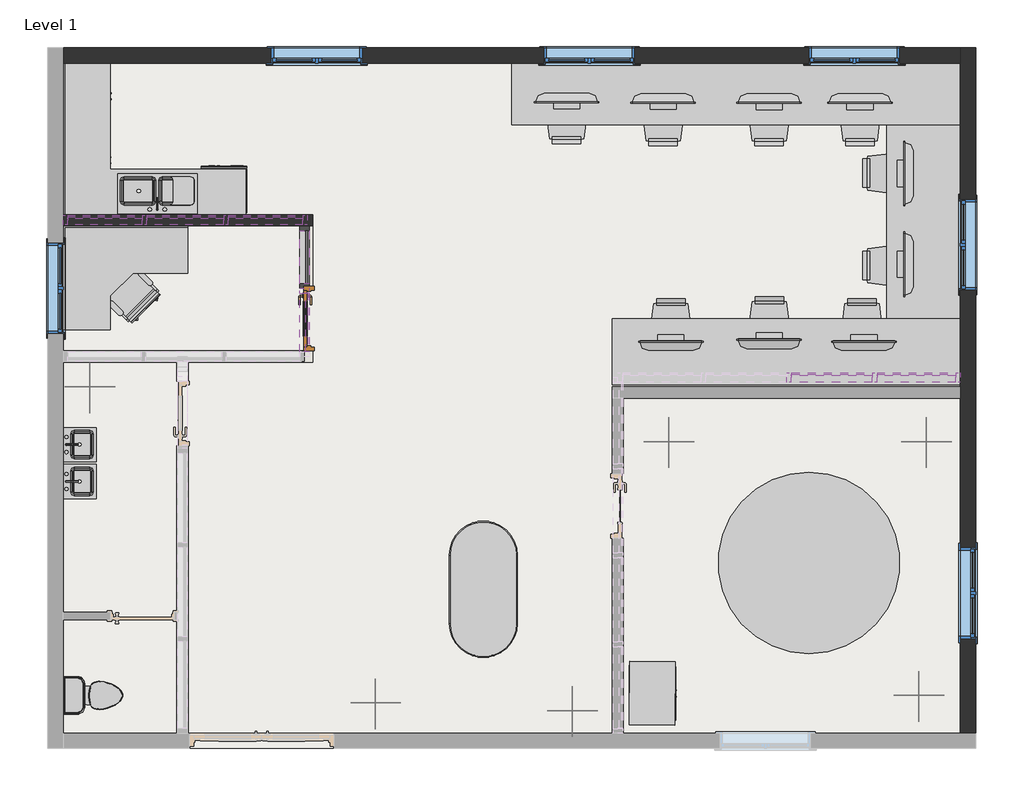
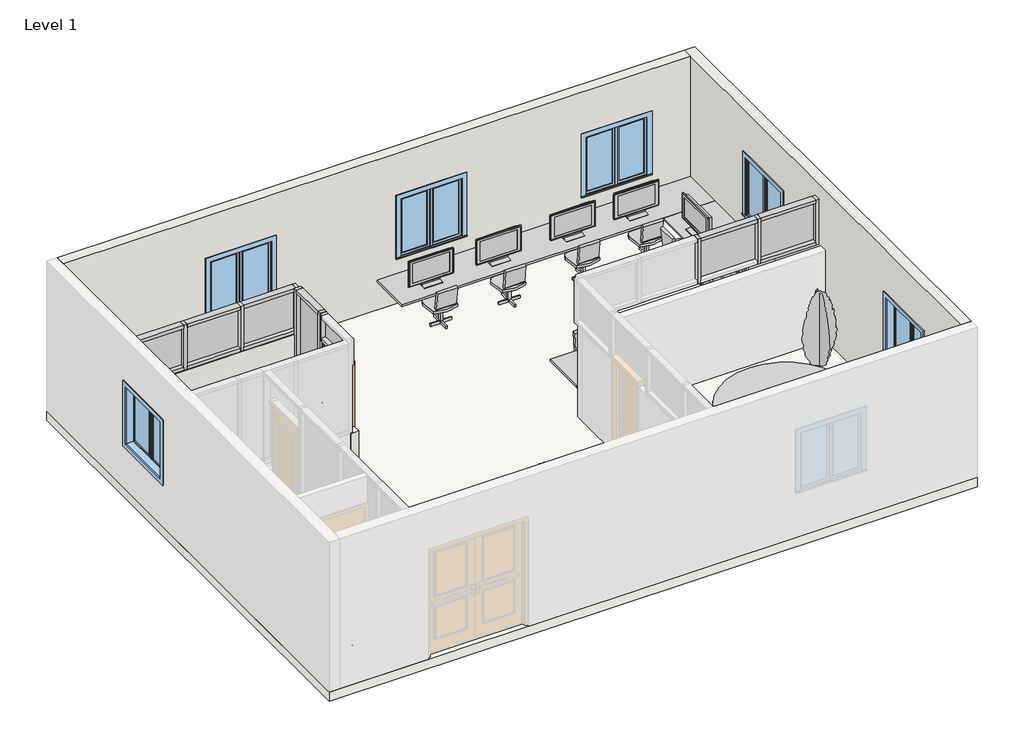
# One storey, part 2 of 2: 30 furniture elements, 22 members, 7 plates, 6 geographic elements, 6 windows, 4 flow terminals, 4 walls, 1 door, 2 other elements.
"""IFC4 building model written with IfcOpenShell, lengths in millimetres."""

from ifc_helpers import new_model, si_unit, frame, origin, origin_with_axes, place, context, project, spatial, polyline, outline, extrude, faceted_brep, transform, mapped, element, save
from components import proxy_45b28599, door_5d83ff76, flow_terminal_7482ecd1, flow_terminal_871c2e40, toilet_domestic_3d_toilet_domestic_3d_f7549cf7, toilet_domestic_3d_toilet_domestic_3d_183bbd19, furniture_5bfe328f, furniture_2feb49e6, chair_desk_chair_desk_ccc35c8f, chair_task_arms_chair_task_arms_fa5a08ef, furniture_7996aedf, furniture_be580aea, furniture_b7a5125e, counter_top_island_0001_depth_6_5a0cf1da, furniture_96954d7a, furniture_aa189fe6, furniture_56245f3a, furniture_f557e78a, furniture_2c34a4f9, furniture_5d3b8c6f, rpc_tree_conifer_chinese_juniper_7_7598bbdc, member_883d71fc, member_79ceace6, member_410c6227, member_73c23c35, member_7fa39cca, member_95280835, member_ae70dd35, member_429f6687, member_3ffc8328, member_f1b77eba, system_panel_glazed_b223e52b, system_panel_glazed_d348d9e0, system_panel_glazed_cfce8111, system_panel_glazed_768357cb, system_panel_glazed_23071c8f, system_panel_glazed_23dedc8c, window_0862ab64

model = new_model("IFC4")

# Units and contexts
model_context = context("Model", 3, world=origin())
ifc_project = project(units=[si_unit("LENGTHUNIT", "METRE", prefix="MILLI")], contexts=[model_context])

# Site, building, storey
site = spatial("IfcSite", under=ifc_project)
building = spatial("IfcBuilding", under=site)
storey = spatial("IfcBuildingStorey", under=building, Name="Level 1", Elevation=0.0)

# Proxy
placement = place(None, origin())
proxy_shape = proxy_45b28599(model_context)
element("IfcBuildingElementProxy", 1, Name="Dishwasher : 24\" x 24\" x 34\"", ObjectType="Dishwasher : 24\" x 24\" x 34\"", at=placement, inside=storey, context=model_context, shape_type="MappedRepresentation", body=[
    mapped(proxy_shape, transform((7305.6010577, -5794.5703949, 0.0), x_axis=(-1.0000000000000004, 0.0, 0.0), y_axis=(0.0, -1.0000000000000004, 0.0), z_axis=(0.0, 0.0, 1.0))),
])

# Door
door_shape = door_5d83ff76(model_context)
element("IfcDoor", 2, ObjectType="Door-Passage-Single-Full_Lite : 30\" x 84\"", at=placement, inside=storey, context=model_context, shape_type="MappedRepresentation", body=[
    mapped(door_shape, transform((8048.5510577, -7788.7208301, 0.0), x_axis=(0.0, -1.0, 0.0), y_axis=(1.0, 0.0, 0.0), z_axis=(0.0, 0.0, 1.0))),
])

# Flow terminals
flow_terminal_shape = flow_terminal_7482ecd1(model_context)
element("IfcFlowTerminal", 3, ObjectType="Sink Kitchen-Double : 42\" x 21\"", at=placement, inside=storey, context=model_context, shape_type="MappedRepresentation", body=[
    mapped(flow_terminal_shape, transform((6013.16127, -6109.9754289, 0.0), x_axis=(1.0000000000000002, 0.0, 0.0), y_axis=(0.0, 1.0000000000000002, 0.0), z_axis=(0.0, 0.0, 1.0))),
])
flow_terminal_2_shape = flow_terminal_871c2e40(model_context)
element("IfcFlowTerminal", 4, ObjectType="Sink Kitchen-Island : 18\" x 18\"", at=placement, inside=storey, context=model_context, shape_type="MappedRepresentation", body=[
    mapped(flow_terminal_2_shape, transform((4983.8464589, -9493.5100706, 0.0), x_axis=(0.0, 1.0000000000000002, 0.0), y_axis=(-1.0000000000000002, 0.0, 0.0), z_axis=(0.0, 0.0, 1.0))),
])
element("IfcFlowTerminal", 5, ObjectType="Sink Kitchen-Island : 18\" x 18\"", at=placement, inside=storey, context=model_context, shape_type="MappedRepresentation", body=[
    mapped(flow_terminal_2_shape, transform((4983.8464589, -9988.8100706, 0.0), x_axis=(0.0, 1.0000000000000002, 0.0), y_axis=(-1.0000000000000002, 0.0, 0.0), z_axis=(0.0, 0.0, 1.0))),
])
toilet_domestic_3d_toilet_domestic_3d_shape = toilet_domestic_3d_toilet_domestic_3d_f7549cf7(model_context)
toilet_domestic_3d_toilet_domestic_3d_2_shape = toilet_domestic_3d_toilet_domestic_3d_183bbd19(model_context)
element("IfcFlowTerminal", 6, ObjectType="Toilet-Domestic-3D : Toilet-Domestic-3D", at=placement, inside=storey, context=model_context, shape_type="MappedRepresentation", body=[
    mapped(toilet_domestic_3d_toilet_domestic_3d_shape, transform((5260.2970851, -12843.3208301, 0.0), x_axis=(0.0, 1.0000000000000002, 0.0), y_axis=(-1.0000000000000002, 0.0, 0.0), z_axis=(0.0, 0.0, 1.0))),
    mapped(toilet_domestic_3d_toilet_domestic_3d_2_shape, transform((5260.2970851, -12843.3208301, 0.0), x_axis=(0.0, 1.0000000000000002, 0.0), y_axis=(-1.0000000000000002, 0.0, 0.0), z_axis=(0.0, 0.0, 1.0))),
])

# Furniture
furniture_shape = furniture_5bfe328f(model_context)
element("IfcFurniture", 7, ObjectType="Base Cabinet-Double Door Sink Unit : 30\"", at=placement, inside=storey, context=model_context, shape_type="MappedRepresentation", body=[
    mapped(furniture_shape, transform((12360.2010577, -12836.658535, 0.0), x_axis=(0.0, 1.0, 0.0), y_axis=(-1.0, 0.0, 0.0), z_axis=(0.0, 0.0, 1.0))),
])
furniture_2_shape = furniture_2feb49e6(model_context)
element("IfcFurniture", 8, ObjectType="Base Cabinet-Double Door Sink Unit : 30\"", at=placement, inside=storey, context=model_context, shape_type="MappedRepresentation", body=[
    mapped(furniture_2_shape, transform((4778.3010577, -4785.4831251, 0.0), x_axis=(0.0, -1.0, 0.0), y_axis=(1.0, 0.0, 0.0), z_axis=(0.0, 0.0, 1.0))),
])
element("IfcFurniture", 9, ObjectType="Base Cabinet-Double Door Sink Unit : 30\"", at=placement, inside=storey, context=model_context, shape_type="MappedRepresentation", body=[
    mapped(furniture_2_shape, transform((4770.3578387, -5644.7380576, 0.0), x_axis=(0.0, -1.0, 0.0), y_axis=(1.0, 0.0, 0.0), z_axis=(0.0, 0.0, 1.0))),
])
chair_desk_chair_desk_shape = chair_desk_chair_desk_ccc35c8f(model_context)
element("IfcFurniture", 10, ObjectType="Chair-Desk : Chair-Desk", at=placement, inside=storey, context=model_context, shape_type="MappedRepresentation", body=[
    mapped(chair_desk_chair_desk_shape, transform((11522.0010577, -5375.7208301, 0.0), x_axis=(1.0, 0.0, 0.0), y_axis=(0.0, 1.0, 0.0), z_axis=(0.0, 0.0, 1.0))),
])
element("IfcFurniture", 11, ObjectType="Chair-Desk : Chair-Desk", at=placement, inside=storey, context=model_context, shape_type="MappedRepresentation", body=[
    mapped(chair_desk_chair_desk_shape, transform((12817.4010577, -5401.1208301, 0.0), x_axis=(1.0, 0.0, 0.0), y_axis=(0.0, 1.0, 0.0), z_axis=(0.0, 0.0, 1.0))),
])
element("IfcFurniture", 12, ObjectType="Chair-Desk : Chair-Desk", at=placement, inside=storey, context=model_context, shape_type="MappedRepresentation", body=[
    mapped(chair_desk_chair_desk_shape, transform((14239.8010577, -5401.1208301, 0.0), x_axis=(1.0, 0.0, 0.0), y_axis=(0.0, 1.0, 0.0), z_axis=(0.0, 0.0, 1.0))),
])
element("IfcFurniture", 13, ObjectType="Chair-Desk : Chair-Desk", at=placement, inside=storey, context=model_context, shape_type="MappedRepresentation", body=[
    mapped(chair_desk_chair_desk_shape, transform((15459.0010577, -5401.1208301, 0.0), x_axis=(1.0, 0.0, 0.0), y_axis=(0.0, 1.0, 0.0), z_axis=(0.0, 0.0, 1.0))),
])
element("IfcFurniture", 14, ObjectType="Chair-Desk : Chair-Desk", at=placement, inside=storey, context=model_context, shape_type="MappedRepresentation", body=[
    mapped(chair_desk_chair_desk_shape, transform((12919.0010577, -7585.5208301, 0.0), x_axis=(-1.0000000000000004, 0.0, 0.0), y_axis=(0.0, -1.0000000000000004, 0.0), z_axis=(0.0, 0.0, 1.0))),
])
element("IfcFurniture", 15, ObjectType="Chair-Desk : Chair-Desk", at=placement, inside=storey, context=model_context, shape_type="MappedRepresentation", body=[
    mapped(chair_desk_chair_desk_shape, transform((14239.8010577, -7560.1208301, 0.0), x_axis=(-1.0, 0.0, 0.0), y_axis=(0.0, -1.0, 0.0), z_axis=(0.0, 0.0, 1.0))),
])
element("IfcFurniture", 16, ObjectType="Chair-Desk : Chair-Desk", at=placement, inside=storey, context=model_context, shape_type="MappedRepresentation", body=[
    mapped(chair_desk_chair_desk_shape, transform((15484.4010577, -7585.5208301, 0.0), x_axis=(-1.0, 0.0, 0.0), y_axis=(0.0, -1.0, 0.0), z_axis=(0.0, 0.0, 1.0))),
])
element("IfcFurniture", 17, ObjectType="Chair-Desk : Chair-Desk", at=placement, inside=storey, context=model_context, shape_type="MappedRepresentation", body=[
    mapped(chair_desk_chair_desk_shape, transform((15560.6010577, -5839.0589124, 0.0), x_axis=(0.0, -1.0, 0.0), y_axis=(1.0, 0.0, 0.0), z_axis=(0.0, 0.0, 1.0))),
])
element("IfcFurniture", 18, ObjectType="Chair-Desk : Chair-Desk", at=placement, inside=storey, context=model_context, shape_type="MappedRepresentation", body=[
    mapped(chair_desk_chair_desk_shape, transform((15560.6010577, -7077.5208301, 0.0), x_axis=(0.0, -1.0, 0.0), y_axis=(1.0, 0.0, 0.0), z_axis=(0.0, 0.0, 1.0))),
])
chair_task_arms_chair_task_arms_shape = chair_task_arms_chair_task_arms_fa5a08ef(model_context)
element("IfcFurniture", 19, ObjectType="Chair-Task Arms : Chair-Task Arms", at=placement, inside=storey, context=model_context, shape_type="MappedRepresentation", body=[
    mapped(chair_task_arms_chair_task_arms_shape, transform((5604.5330031, -7582.4439048, 0.0), x_axis=(0.7071067811865507, 0.7071067811865445, 0.0), y_axis=(-0.7071067811865445, 0.7071067811865507, 0.0), z_axis=(0.0, 0.0, 1.0))),
])
furniture_3_shape = furniture_7996aedf(model_context)
element("IfcFurniture", 20, ObjectType="Counter Top-Island : 48\" Depth", at=placement, inside=storey, context=model_context, shape_type="MappedRepresentation", body=[
    mapped(furniture_3_shape, transform((12955.5284008, -12044.4840518, 0.0), x_axis=(0.008496168549226357, 0.999963906908636, 0.0), y_axis=(-0.999963906908636, 0.008496168549226357, 0.0), z_axis=(0.0, 0.0, 1.0))),
])
furniture_4_shape = furniture_be580aea(model_context)
element("IfcFurniture", 21, ObjectType="Counter Top-Island.0001 : 48\" Depth", at=placement, inside=storey, context=model_context, shape_type="MappedRepresentation", body=[
    mapped(furniture_4_shape, transform((15839.7435195, -6588.258535, 0.0), x_axis=(0.0, 1.0000000000000002, 0.0), y_axis=(-1.0000000000000002, 0.0, 0.0), z_axis=(0.0, 0.0, 1.0))),
])
furniture_5_shape = furniture_b7a5125e(model_context)
element("IfcFurniture", 22, ObjectType="Counter Top-Island.0001 : 48\" Depth", at=placement, inside=storey, context=model_context, shape_type="MappedRepresentation", body=[
    mapped(furniture_5_shape, transform((11985.8633528, -4359.7208301, 0.0), x_axis=(1.0, 0.0, 0.0), y_axis=(0.0, 1.0, 0.0), z_axis=(0.0, 0.0, 1.0))),
])
counter_top_island_0001_depth_6_shape = counter_top_island_0001_depth_6_5a0cf1da(model_context)
element("IfcFurniture", 23, ObjectType="Counter Top-Island.0001 : depth 6'", at=placement, inside=storey, context=model_context, shape_type="MappedRepresentation", body=[
    mapped(counter_top_island_0001_depth_6_shape, transform((13332.0633528, -8652.3208301, 0.0), x_axis=(1.0, 0.0, 0.0), y_axis=(0.0, 1.0, 0.0), z_axis=(0.0, 0.0, 1.0))),
])
furniture_6_shape = furniture_96954d7a(model_context)
element("IfcFurniture", 24, ObjectType="Counter Top-L Shaped 2 : 24\" Depth", at=placement, inside=storey, context=model_context, shape_type="MappedRepresentation", body=[
    mapped(furniture_6_shape, transform((5966.0633528, -6544.1208301, 0.0), x_axis=(1.0, 0.0, 0.0), y_axis=(0.0, 1.0, 0.0), z_axis=(0.0, 0.0, 1.0))),
])
furniture_7_shape = furniture_aa189fe6(model_context)
element("IfcFurniture", 25, ObjectType="Counter Top-L Shaped w Sink : 24\" Depth", at=placement, inside=storey, context=model_context, shape_type="MappedRepresentation", body=[
    mapped(furniture_7_shape, transform((5966.0633528, -6417.1208301, 0.0), x_axis=(1.0000000000000002, 0.0, 0.0), y_axis=(0.0, 1.0000000000000002, 0.0), z_axis=(0.0, 0.0, 1.0))),
])
furniture_8_shape = furniture_56245f3a(model_context)
element("IfcFurniture", 26, ObjectType="TV - Flat Screen : 32\"", at=placement, inside=storey, context=model_context, shape_type="MappedRepresentation", body=[
    mapped(furniture_8_shape, transform((14243.7455719, -4830.797536, 609.6), x_axis=(1.0, 0.0, 0.0), y_axis=(0.0, 1.0, 0.0), z_axis=(0.0, 0.0, 1.0))),
])
element("IfcFurniture", 27, ObjectType="TV - Flat Screen : 32\"", at=placement, inside=storey, context=model_context, shape_type="MappedRepresentation", body=[
    mapped(furniture_8_shape, transform((12821.3455719, -4830.3773567, 609.6), x_axis=(1.0, 0.0, 0.0), y_axis=(0.0, 1.0, 0.0), z_axis=(0.0, 0.0, 1.0))),
])
element("IfcFurniture", 28, ObjectType="TV - Flat Screen : 32\"", at=placement, inside=storey, context=model_context, shape_type="MappedRepresentation", body=[
    mapped(furniture_8_shape, transform((11525.9455719, -4823.6359141, 609.6), x_axis=(1.0, 0.0, 0.0), y_axis=(0.0, 1.0, 0.0), z_axis=(0.0, 0.0, 1.0))),
])
element("IfcFurniture", 29, ObjectType="TV - Flat Screen : 32\"", at=placement, inside=storey, context=model_context, shape_type="MappedRepresentation", body=[
    mapped(furniture_8_shape, transform((16111.6624341, -5843.0034265, 609.6), x_axis=(0.0, -1.0000000000000007, 0.0), y_axis=(1.0000000000000007, 0.0, 0.0), z_axis=(0.0, 0.0, 1.0))),
])
element("IfcFurniture", 30, ObjectType="TV - Flat Screen : 32\"", at=placement, inside=storey, context=model_context, shape_type="MappedRepresentation", body=[
    mapped(furniture_8_shape, transform((15462.9455719, -4830.797536, 609.6), x_axis=(1.0, 0.0, 0.0), y_axis=(0.0, 1.0, 0.0), z_axis=(0.0, 0.0, 1.0))),
])
element("IfcFurniture", 31, ObjectType="TV - Flat Screen : 32\"", at=placement, inside=storey, context=model_context, shape_type="MappedRepresentation", body=[
    mapped(furniture_8_shape, transform((16111.6624341, -7062.2034265, 609.6), x_axis=(0.0, -1.0000000000000007, 0.0), y_axis=(1.0000000000000007, 0.0, 0.0), z_axis=(0.0, 0.0, 1.0))),
])
furniture_9_shape = furniture_f557e78a(model_context)
element("IfcFurniture", 32, ObjectType="TV - Flat Screen : 32\"", at=placement, inside=storey, context=model_context, shape_type="MappedRepresentation", body=[
    mapped(furniture_9_shape, transform((15513.7455719, -8155.8441241, 609.6), x_axis=(1.0, 0.0, 0.0), y_axis=(0.0, 1.0, 0.0), z_axis=(0.0, 0.0, 1.0))),
])
element("IfcFurniture", 33, ObjectType="TV - Flat Screen : 32\"", at=placement, inside=storey, context=model_context, shape_type="MappedRepresentation", body=[
    mapped(furniture_9_shape, transform((14243.7455719, -8130.4441241, 609.6), x_axis=(1.0, 0.0, 0.0), y_axis=(0.0, 1.0, 0.0), z_axis=(0.0, 0.0, 1.0))),
])
element("IfcFurniture", 34, ObjectType="TV - Flat Screen : 32\"", at=placement, inside=storey, context=model_context, shape_type="MappedRepresentation", body=[
    mapped(furniture_9_shape, transform((12922.9455719, -8156.2643034, 609.6), x_axis=(1.0, 0.0, 0.0), y_axis=(0.0, 1.0, 0.0), z_axis=(0.0, 0.0, 1.0))),
])
furniture_10_shape = furniture_2c34a4f9(model_context)
element("IfcFurniture", 35, ObjectType="Table-Dining Oval : 36\" x 72\"", at=placement, inside=storey, context=model_context, shape_type="MappedRepresentation", body=[
    mapped(furniture_10_shape, transform((10046.3026971, -11019.1011579, 0.0), x_axis=(0.0, 1.0, 0.0), y_axis=(-1.0, 0.0, 0.0), z_axis=(0.0, 0.0, 1.0))),
])
furniture_11_shape = furniture_5d3b8c6f(model_context)
element("IfcFurniture", 36, ObjectType="Table-Dining Round w Chairs : 36\" Diameter", at=placement, inside=storey, context=model_context, shape_type="MappedRepresentation", body=[
    mapped(furniture_11_shape, transform((14669.5190905, -10880.4421415, 0.0), x_axis=(1.0, 0.0, 0.0), y_axis=(0.0, 1.0, 0.0), z_axis=(0.0, 0.0, 1.0))),
])

# Geographic elements
rpc_tree_conifer_chinese_juniper_7_shape = rpc_tree_conifer_chinese_juniper_7_7598bbdc(model_context)
element("IfcGeographicElement", 37, ObjectType="RPC Tree - Conifer : Chinese Juniper - 7'", at=placement, inside=storey, context=model_context, shape_type="MappedRepresentation", body=[
    mapped(rpc_tree_conifer_chinese_juniper_7_shape, transform((16347.8043867, -9439.7208301, 0.0), x_axis=(1.0, 0.0, 0.0), y_axis=(0.0, 1.0, 0.0), z_axis=(0.0, 0.0, 1.0))),
])
element("IfcGeographicElement", 38, ObjectType="RPC Tree - Conifer : Chinese Juniper - 7'", at=placement, inside=storey, context=model_context, shape_type="MappedRepresentation", body=[
    mapped(rpc_tree_conifer_chinese_juniper_7_shape, transform((12893.4043867, -9439.7208301, 0.0), x_axis=(1.0, 0.0, 0.0), y_axis=(0.0, 1.0, 0.0), z_axis=(0.0, 0.0, 1.0))),
])
element("IfcGeographicElement", 39, ObjectType="RPC Tree - Conifer : Chinese Juniper - 7'", at=placement, inside=storey, context=model_context, shape_type="MappedRepresentation", body=[
    mapped(rpc_tree_conifer_chinese_juniper_7_shape, transform((16246.2043867, -12843.3208301, 0.0), x_axis=(1.0, 0.0, 0.0), y_axis=(0.0, 1.0, 0.0), z_axis=(0.0, 0.0, 1.0))),
])
element("IfcGeographicElement", 40, ObjectType="RPC Tree - Conifer : Chinese Juniper - 7'", at=placement, inside=storey, context=model_context, shape_type="MappedRepresentation", body=[
    mapped(rpc_tree_conifer_chinese_juniper_7_shape, transform((5121.0043867, -8703.1208301, 0.0), x_axis=(1.0, 0.0, 0.0), y_axis=(0.0, 1.0, 0.0), z_axis=(0.0, 0.0, 1.0))),
])
element("IfcGeographicElement", 41, ObjectType="RPC Tree - Conifer : Chinese Juniper - 7'", at=placement, inside=storey, context=model_context, shape_type="MappedRepresentation", body=[
    mapped(rpc_tree_conifer_chinese_juniper_7_shape, transform((8956.4043867, -12944.9208301, 0.0), x_axis=(1.0, 0.0, 0.0), y_axis=(0.0, 1.0, 0.0), z_axis=(0.0, 0.0, 1.0))),
])
element("IfcGeographicElement", 42, ObjectType="RPC Tree - Conifer : Chinese Juniper - 7'", at=placement, inside=storey, context=model_context, shape_type="MappedRepresentation", body=[
    mapped(rpc_tree_conifer_chinese_juniper_7_shape, transform((11598.0043867, -13046.5208301, 0.0), x_axis=(1.0, 0.0, 0.0), y_axis=(0.0, 1.0, 0.0), z_axis=(0.0, 0.0, 1.0))),
])

# Members
member_shape = member_883d71fc(model_context)
element("IfcMember", 43, ObjectType="Rectangular Mullion : 2.5\" x 5\" rectangular", at=placement, inside=storey, context=model_context, shape_type="MappedRepresentation", body=[
    mapped(member_shape, transform((7978.7010577, -6467.9208301, 2743.2), x_axis=(0.0, 0.0, 1.0), y_axis=(0.0, -1.0, 0.0), z_axis=(1.0, 0.0, 0.0))),
])
element("IfcMember", 44, ObjectType="Rectangular Mullion : 2.5\" x 5\" rectangular", at=placement, inside=storey, context=model_context, shape_type="MappedRepresentation", body=[
    mapped(member_shape, transform((5826.0510577, -6467.9208301, 2743.2), x_axis=(0.0, 0.0, 1.0), y_axis=(0.0, -1.0, 0.0), z_axis=(1.0, 0.0, 0.0))),
])
member_2_shape = member_79ceace6(model_context)
element("IfcMember", 45, ObjectType="Rectangular Mullion : 2.5\" x 5\" rectangular", at=placement, inside=storey, context=model_context, shape_type="MappedRepresentation", body=[
    mapped(member_2_shape, transform((6918.2510577, -6467.9208301, 2743.2), x_axis=(0.0, 0.0, 1.0), y_axis=(0.0, -1.0, 0.0), z_axis=(1.0, 0.0, 0.0))),
])
element("IfcMember", 46, ObjectType="Rectangular Mullion : 2.5\" x 5\" rectangular", at=placement, inside=storey, context=model_context, shape_type="MappedRepresentation", body=[
    mapped(member_shape, transform((4829.1010577, -6467.9208301, 1828.8), x_axis=(0.0, 0.0, -1.0), y_axis=(0.0, -1.0, 0.0), z_axis=(-1.0, 0.0, 0.0))),
])
element("IfcMember", 47, ObjectType="Rectangular Mullion : 2.5\" x 5\" rectangular", at=placement, inside=storey, context=model_context, shape_type="MappedRepresentation", body=[
    mapped(member_shape, transform((6981.7510577, -6467.9208301, 1828.8), x_axis=(0.0, 0.0, -1.0), y_axis=(0.0, -1.0, 0.0), z_axis=(-1.0, 0.0, 0.0))),
])
element("IfcMember", 48, ObjectType="Rectangular Mullion : 2.5\" x 5\" rectangular", at=placement, inside=storey, context=model_context, shape_type="MappedRepresentation", body=[
    mapped(member_2_shape, transform((5889.5510577, -6467.9208301, 1828.8), x_axis=(0.0, 0.0, -1.0), y_axis=(0.0, -1.0, 0.0), z_axis=(-1.0, 0.0, 0.0))),
])
member_3_shape = member_410c6227(model_context)
element("IfcMember", 49, ObjectType="Rectangular Mullion : 2.5\" x 5\" rectangular", at=placement, inside=storey, context=model_context, shape_type="MappedRepresentation", body=[
    mapped(member_3_shape, transform((5857.8010577, -6467.9208301, 1828.8), x_axis=(1.0, 0.0, 0.0), y_axis=(0.0, -1.0, 0.0), z_axis=(0.0, 0.0, -1.0))),
])
element("IfcMember", 50, ObjectType="Rectangular Mullion : 2.5\" x 5\" rectangular", at=placement, inside=storey, context=model_context, shape_type="MappedRepresentation", body=[
    mapped(member_3_shape, transform((6950.0010577, -6467.9208301, 1828.8), x_axis=(1.0, 0.0, 0.0), y_axis=(0.0, -1.0, 0.0), z_axis=(0.0, 0.0, -1.0))),
])
element("IfcMember", 51, ObjectType="Rectangular Mullion : 2.5\" x 5\" rectangular", at=placement, inside=storey, context=model_context, shape_type="MappedRepresentation", body=[
    mapped(member_3_shape, transform((14506.5010577, -8576.1208301, 1828.8), x_axis=(1.0, 0.0, 0.0), y_axis=(0.0, -1.0, 0.0), z_axis=(0.0, 0.0, -1.0))),
])
element("IfcMember", 52, ObjectType="Rectangular Mullion : 2.5\" x 5\" rectangular", at=placement, inside=storey, context=model_context, shape_type="MappedRepresentation", body=[
    mapped(member_3_shape, transform((15655.8510577, -8576.1208301, 1828.8), x_axis=(1.0, 0.0, 0.0), y_axis=(0.0, -1.0, 0.0), z_axis=(0.0, 0.0, -1.0))),
])
member_4_shape = member_73c23c35(model_context)
element("IfcMember", 53, ObjectType="Rectangular Mullion : 2.5\" x 5\" rectangular", at=placement, inside=storey, context=model_context, shape_type="MappedRepresentation", body=[
    mapped(member_4_shape, transform((8042.2010577, -6467.9208301, 1828.8), x_axis=(1.0, 0.0, 0.0), y_axis=(0.0, -1.0, 0.0), z_axis=(0.0, 0.0, -1.0))),
])
element("IfcMember", 54, ObjectType="Rectangular Mullion : 2.5\" x 5\" rectangular", at=placement, inside=storey, context=model_context, shape_type="MappedRepresentation", body=[
    mapped(member_4_shape, transform((16805.2010577, -8576.1208301, 1828.8), x_axis=(1.0, 0.0, 0.0), y_axis=(0.0, -1.0, 0.0), z_axis=(0.0, 0.0, -1.0))),
])
element("IfcMember", 55, ObjectType="Rectangular Mullion : 2.5\" x 5\" rectangular", at=placement, inside=storey, context=model_context, shape_type="MappedRepresentation", body=[
    mapped(member_4_shape, transform((4765.6010577, -6467.9208301, 2743.2), x_axis=(-1.0, 0.0, 0.0), y_axis=(0.0, -1.0, 0.0), z_axis=(0.0, 0.0, 1.0))),
])
member_5_shape = member_7fa39cca(model_context)
element("IfcMember", 56, ObjectType="Rectangular Mullion : 2.5\" x 5\" rectangular", at=placement, inside=storey, context=model_context, shape_type="MappedRepresentation", body=[
    mapped(member_5_shape, transform((16741.7010577, -8576.1208301, 2743.2), x_axis=(0.0, 0.0, 1.0), y_axis=(0.0, -1.0, 0.0), z_axis=(1.0, 0.0, 0.0))),
])
member_6_shape = member_95280835(model_context)
element("IfcMember", 57, ObjectType="Rectangular Mullion : 2.5\" x 5\" rectangular", at=placement, inside=storey, context=model_context, shape_type="MappedRepresentation", body=[
    mapped(member_6_shape, transform((15624.1010577, -8576.1208301, 2743.2), x_axis=(0.0, 0.0, 1.0), y_axis=(0.0, -1.0, 0.0), z_axis=(1.0, 0.0, 0.0))),
])
element("IfcMember", 58, ObjectType="Rectangular Mullion : 2.5\" x 5\" rectangular", at=placement, inside=storey, context=model_context, shape_type="MappedRepresentation", body=[
    mapped(member_5_shape, transform((15687.6010577, -8576.1208301, 1828.8), x_axis=(0.0, 0.0, -1.0), y_axis=(0.0, -1.0, 0.0), z_axis=(-1.0, 0.0, 0.0))),
])
member_7_shape = member_ae70dd35(model_context)
element("IfcMember", 59, ObjectType="Rectangular Mullion : 2.5\" x 5\" rectangular", at=placement, inside=storey, context=model_context, shape_type="MappedRepresentation", body=[
    mapped(member_7_shape, transform((8004.1010577, -7318.8208301, 2764.3041833), x_axis=(0.0, 0.0, 1.0), y_axis=(-1.0, 0.0, 0.0), z_axis=(0.0, -1.0, 0.0))),
])
element("IfcMember", 60, ObjectType="Rectangular Mullion : 2.5\" x 5\" rectangular", at=placement, inside=storey, context=model_context, shape_type="MappedRepresentation", body=[
    mapped(member_7_shape, transform((8004.1010577, -6607.6208301, 914.4), x_axis=(0.0, 0.0, -1.0), y_axis=(-1.0, 0.0, 0.0), z_axis=(0.0, 1.0, 0.0))),
])
member_8_shape = member_429f6687(model_context)
element("IfcMember", 61, ObjectType="Rectangular Mullion : 2.5\" x 5\" rectangular", at=placement, inside=storey, context=model_context, shape_type="MappedRepresentation", body=[
    mapped(member_8_shape, transform((8004.1010577, -7445.8208301, 2235.2), x_axis=(0.0, 0.0, -1.0), y_axis=(-1.0, 0.0, 0.0), z_axis=(0.0, 1.0, 0.0))),
])
member_9_shape = member_3ffc8328(model_context)
element("IfcMember", 62, ObjectType="Rectangular Mullion : 2.5\" x 5\" rectangular", at=placement, inside=storey, context=model_context, shape_type="MappedRepresentation", body=[
    mapped(member_9_shape, transform((8004.1010577, -7382.3208301, 914.4), x_axis=(0.0, -1.0, 0.0), y_axis=(-1.0, 0.0, 0.0), z_axis=(0.0, 0.0, -1.0))),
])
element("IfcMember", 63, ObjectType="Rectangular Mullion : 2.5\" x 5\" rectangular", at=placement, inside=storey, context=model_context, shape_type="MappedRepresentation", body=[
    mapped(member_9_shape, transform((8004.1010577, -6544.1208301, 2764.3041833), x_axis=(0.0, 1.0, 0.0), y_axis=(-1.0, 0.0, 0.0), z_axis=(0.0, 0.0, 1.0))),
])
member_10_shape = member_f1b77eba(model_context)
element("IfcMember", 64, ObjectType="Rectangular Mullion : 2.5\" x 5\" rectangular", at=placement, inside=storey, context=model_context, shape_type="MappedRepresentation", body=[
    mapped(member_10_shape, transform((8004.1010577, -7382.3208301, 2754.1090709), x_axis=(0.0, 1.0, 0.0), y_axis=(-1.0, 0.0, 0.0), z_axis=(0.0, 0.0, 1.0))),
])

# Plates
system_panel_glazed_shape = system_panel_glazed_b223e52b(model_context)
element("IfcPlate", 65, ObjectType="System Panel : Glazed", at=placement, inside=storey, context=model_context, shape_type="MappedRepresentation", body=[
    mapped(system_panel_glazed_shape, transform((5327.5760577, -6467.9208301, 1892.3), x_axis=(1.0, 0.0, 0.0), y_axis=(0.0, 1.0, 0.0), z_axis=(0.0, 0.0, 1.0))),
])
element("IfcPlate", 66, ObjectType="System Panel : Glazed", at=placement, inside=storey, context=model_context, shape_type="MappedRepresentation", body=[
    mapped(system_panel_glazed_shape, transform((7480.2260577, -6467.9208301, 1892.3), x_axis=(1.0, 0.0, 0.0), y_axis=(0.0, 1.0, 0.0), z_axis=(0.0, 0.0, 1.0))),
])
system_panel_glazed_2_shape = system_panel_glazed_d348d9e0(model_context)
element("IfcPlate", 67, ObjectType="System Panel : Glazed", at=placement, inside=storey, context=model_context, shape_type="MappedRepresentation", body=[
    mapped(system_panel_glazed_2_shape, transform((6403.9010577, -6467.9208301, 1892.3), x_axis=(1.0, 0.0, 0.0), y_axis=(0.0, 1.0, 0.0), z_axis=(0.0, 0.0, 1.0))),
])
system_panel_glazed_3_shape = system_panel_glazed_cfce8111(model_context)
element("IfcPlate", 68, ObjectType="System Panel : Glazed", at=placement, inside=storey, context=model_context, shape_type="MappedRepresentation", body=[
    mapped(system_panel_glazed_3_shape, transform((16214.6510577, -8576.1208301, 1892.3), x_axis=(1.0, 0.0, 0.0), y_axis=(0.0, 1.0, 0.0), z_axis=(0.0, 0.0, 1.0))),
])
system_panel_glazed_4_shape = system_panel_glazed_768357cb(model_context)
element("IfcPlate", 69, ObjectType="System Panel : Glazed", at=placement, inside=storey, context=model_context, shape_type="MappedRepresentation", body=[
    mapped(system_panel_glazed_4_shape, transform((15081.1760577, -8576.1208301, 1892.3), x_axis=(1.0, 0.0, 0.0), y_axis=(0.0, 1.0, 0.0), z_axis=(0.0, 0.0, 1.0))),
])
system_panel_glazed_5_shape = system_panel_glazed_23071c8f(model_context)
element("IfcPlate", 70, ObjectType="System Panel : Glazed", at=placement, inside=storey, context=model_context, shape_type="MappedRepresentation", body=[
    mapped(system_panel_glazed_5_shape, transform((8004.1010577, -6963.2208301, 977.9), x_axis=(0.0, -1.0, 0.0), y_axis=(1.0, 0.0, 0.0), z_axis=(0.0, 0.0, 1.0))),
])
system_panel_glazed_6_shape = system_panel_glazed_23dedc8c(model_context)
element("IfcPlate", 71, ObjectType="System Panel : Glazed", at=placement, inside=storey, context=model_context, shape_type="MappedRepresentation", body=[
    mapped(system_panel_glazed_6_shape, transform((8004.1010577, -7839.5208301, 2298.7), x_axis=(0.0, -1.0, 0.0), y_axis=(1.0, 0.0, 0.0), z_axis=(0.0, 0.0, 1.0))),
])

# Slab
element("IfcSlab", 72, ObjectType="Generic - 12\"", at=placement, inside=storey, context=model_context, shape_type="SweptSolid", body=[
    extrude(outline(polyline([(17008.4010577, -4156.5208301), (17008.4010577, -13554.5208301), (4562.4010577, -13554.5208301), (4562.4010577, -4156.5208301), (17008.4010577, -4156.5208301)])), frame((0.0, 0.0, -182.8601563), z_axis=(0.0, 0.0, 1.0), x_axis=(1.0, 0.0, 0.0)), (0.0, 0.0, 1.0), 182.8601563),
])

# Walls
element("IfcWall", 73, ObjectType="Generic - 6\"", at=placement, inside=storey, context=model_context, shape_type="Brep", body=[
    faceted_brep([(4765.6010577, -6544.1208301, 0.0), (7966.0010577, -6544.1208301, 0.0), (8118.4010577, -6544.1208301, 0.0), (8118.4010577, -6544.1208301, 914.4), (8118.4010577, -6544.1208301, 1828.8), (4765.6010577, -6544.1208301, 1828.8), (4765.6010577, -6391.7208301, 0.0), (4765.6010577, -6391.7208301, 1828.8), (8118.4010577, -6391.7208301, 1828.8), (8118.4010577, -6391.7208301, 0.0)], [[[0, 1, 2, 3, 4, 5]], [[6, 7, 8, 9]], [[2, 1, 0, 6, 9]], [[5, 4, 8, 7]], [[0, 5, 7, 6]], [[4, 3, 2, 9, 8]]]),
])
element("IfcWall", 74, ObjectType="Generic - 6\"", at=placement, inside=storey, context=model_context, shape_type="SweptSolid", body=[
    extrude(outline(polyline([(7966.0010577, -6544.1208301), (8118.4010577, -6544.1208301), (8118.4010577, -7356.9208301), (7966.0010577, -7356.9208301), (7966.0010577, -6544.1208301)])), origin_with_axes(), (0.0, 0.0, 1.0), 914.4),
    extrude(outline(polyline([(8118.4010577, -8372.9208301), (7966.0010577, -8372.9208301), (7966.0010577, -8220.5208301), (8118.4010577, -8220.5208301), (8118.4010577, -8372.9208301)])), origin_with_axes(), (0.0, 0.0, 1.0), 914.4),
])
element("IfcWall", 75, ObjectType="Generic - 8\"", at=placement, inside=storey, context=model_context, shape_type="Brep", body=[
    faceted_brep([(17008.4010577, -13351.3208301, 0.0), (17008.4010577, -4156.5208301, 0.0), (17008.4010577, -4156.5208301, 3048.0), (17008.4010577, -13351.3208301, 3048.0), (17008.4010577, -6188.5208301, 2133.6), (17008.4010577, -6188.5208301, 914.4), (17008.4010577, -7407.7208301, 914.4), (17008.4010577, -7407.7208301, 2133.6), (17008.4010577, -12081.3208301, 2133.6), (17008.4010577, -10862.1208301, 2133.6), (17008.4010577, -10862.1208301, 914.4), (17008.4010577, -12081.3208301, 914.4), (16805.2010577, -13351.3208301, 0.0), (16805.2010577, -13351.3208301, 3048.0), (16805.2010577, -4359.7208301, 3048.0), (16805.2010577, -4156.5208301, 3048.0), (16805.2010577, -4156.5208301, 0.0), (16805.2010577, -4359.7208301, 0.0), (16805.2010577, -8703.1208301, 0.0), (16805.2010577, -8855.5208301, 0.0), (16805.2010577, -6188.5208301, 2133.6), (16805.2010577, -7407.7208301, 2133.6), (16805.2010577, -7407.7208301, 914.4), (16805.2010577, -6188.5208301, 914.4), (16805.2010577, -12081.3208301, 2133.6), (16805.2010577, -12081.3208301, 914.4), (16805.2010577, -10862.1208301, 914.4), (16805.2010577, -10862.1208301, 2133.6)], [[[0, 1, 2, 3], [4, 5, 6, 7], [8, 9, 10, 11]], [[12, 13, 14, 15, 16, 17, 18, 19], [20, 21, 22, 23], [24, 25, 26, 27]], [[1, 0, 12, 19, 18, 17, 16]], [[3, 2, 15, 14, 13]], [[0, 3, 13, 12]], [[2, 1, 16, 15]], [[5, 4, 20, 23]], [[6, 5, 23, 22]], [[7, 6, 22, 21]], [[4, 7, 21, 20]], [[25, 24, 8, 11]], [[26, 25, 11, 10]], [[27, 26, 10, 9]], [[24, 27, 9, 8]]]),
])
element("IfcWall", 76, ObjectType="Generic - 8\"", at=placement, inside=storey, context=model_context, shape_type="SweptSolid", body=[
    extrude(outline(polyline([(0.0, 16805.2010577), (3048.0, 16805.2010577), (3048.0, 4765.6010577), (0.0, 4765.6010577), (0.0, 16805.2010577)]), holes=[polyline([(2133.6, 7559.6010577), (2133.6, 8778.8010577), (914.4, 8778.8010577), (914.4, 7559.6010577), (2133.6, 7559.6010577)]), polyline([(2133.6, 11217.2010577), (2133.6, 12436.4010577), (914.4, 12436.4010577), (914.4, 11217.2010577), (2133.6, 11217.2010577)]), polyline([(2133.6, 14773.2010577), (2133.6, 15992.4010577), (914.4, 15992.4010577), (914.4, 14773.2010577), (2133.6, 14773.2010577)])]), frame((0.0, -4359.7208301, 0.0), z_axis=(0.0, 1.0, 0.0), x_axis=(0.0, 0.0, 1.0)), (0.0, 0.0, 1.0), 203.2),
])

# Windows
window_shape = window_0862ab64(model_context)
element("IfcWindow", 77, ObjectType="Casement Dbl with Trim : 48\" x 48\"", at=placement, inside=storey, context=model_context, shape_type="MappedRepresentation", body=[
    mapped(window_shape, transform((8169.2010577, -4239.0708301, 0.0), x_axis=(-1.0, 0.0, 0.0), y_axis=(0.0, -1.0, 0.0), z_axis=(0.0, 0.0, 1.0))),
])
element("IfcWindow", 78, ObjectType="Casement Dbl with Trim : 48\" x 48\"", at=placement, inside=storey, context=model_context, shape_type="MappedRepresentation", body=[
    mapped(window_shape, transform((11826.8010577, -4239.0708301, 0.0), x_axis=(-1.0, 0.0, 0.0), y_axis=(0.0, -1.0, 0.0), z_axis=(0.0, 0.0, 1.0))),
])
element("IfcWindow", 79, ObjectType="Casement Dbl with Trim : 48\" x 48\"", at=placement, inside=storey, context=model_context, shape_type="MappedRepresentation", body=[
    mapped(window_shape, transform((15382.8010577, -4239.0708301, 0.0), x_axis=(-1.0, 0.0, 0.0), y_axis=(0.0, -1.0, 0.0), z_axis=(0.0, 0.0, 1.0))),
])
element("IfcWindow", 80, ObjectType="Casement Dbl with Trim : 48\" x 48\"", at=placement, inside=storey, context=model_context, shape_type="MappedRepresentation", body=[
    mapped(window_shape, transform((16925.8510577, -6798.1208301, 0.0), x_axis=(0.0, 1.0, 0.0), y_axis=(-1.0, 0.0, 0.0), z_axis=(0.0, 0.0, 1.0))),
])
element("IfcWindow", 81, ObjectType="Casement Dbl with Trim : 48\" x 48\"", at=placement, inside=storey, context=model_context, shape_type="MappedRepresentation", body=[
    mapped(window_shape, transform((16887.7510577, -11471.7208301, 0.0), x_axis=(0.0, -1.0, 0.0), y_axis=(1.0, 0.0, 0.0), z_axis=(0.0, 0.0, 1.0))),
])
element("IfcWindow", 82, ObjectType="Casement Dbl with Trim : 48\" x 48\"", at=placement, inside=storey, context=model_context, shape_type="MappedRepresentation", body=[
    mapped(window_shape, transform((4644.9510577, -7382.3208301, 0.0), x_axis=(0.0, -1.0, 0.0), y_axis=(1.0, 0.0, 0.0), z_axis=(0.0, 0.0, 1.0))),
])

save(model, "model.ifc")

# Revit data of these elements
# Type "Dishwasher : 24\" x 24\" x 34\""
#   Label = "DW"
#   Assembly Code = "E1090400"
#   Depth = 2' - 0"
#   Height = 2' - 10"
#   Width = 2' - 0"
#   Dishwasher Material = Steel, Paint Finish, Ivory, Glossy
#   Panel Face Material = Plastic, Opaque Black
#   Default Elevation = 0
# Type "Door-Passage-Single-Full_Lite : 30\" x 84\""
#   Type Mark = "9"
#   Assembly Code = "B2030100"
#   Analytic Construction = "Wooden"
#   Thickness = 0' - 1 3/4"
#   Thermal Resistance (R) = 2.5876 (h·ft²·°F)/BTU
#   Swing Angle [instance default] = 90.00°
#   Strike Height = 3' - 4"
#   Rough Width [instance default] = 2' - 10"
#   Rough Height [instance default] = 7' - 4"
#   MF Opening Height [instance default] = 0' - 4"
#   MF Opening Width [instance default] = 0' - 4"
#   Inset Calculate [instance default] = 0' - 4"
#   Masonry Inset [instance default] = 0' - 1"
#   Height = 7' - 0"
#   Width = 2' - 6"
#   Heat Transfer Coefficient (U) = 0.3865 BTU/(h·ft²·°F)
#   Masonry Frame Depth = 0' - 5 3/4"
#   Masonry Frame [instance default] = yes
#   Function = 1
#   Dry Wall Frame [instance default] = no
#   Panel Material = Wood - Birch
#   Glazing = Glass
#   Glass Stop Material = Metal - Paint Finish - Grey
#   Frame Material = Metal - Paint Finish - Grey
#   Door Handle Material = Aluminum
#   Visual Light Transmittance = 0
#   Solar Heat Gain Coefficient = 0
#   Wall Closure = (empty or 0)
# Type "Sink Kitchen-Double : 42\" x 21\""
#   Assembly Code = "D2010410"
#   Counter Height = 3' - 0"
#   Depth = 1' - 9"
#   Width = 3' - 6"
#   Faucet Material = Steel, Polished
#   Sink Material = Steel, Polished
#   Default Elevation = 0
# Type "Sink Kitchen-Island : 18\" x 18\""
#   Assembly Code = "D2010410"
#   Counter Height = 3' - 0"
#   Depth = 1' - 6"
#   Width = 1' - 6"
#   Faucet Material = Steel, Polished
#   Sink Material = Steel, Polished
#   Default Elevation = 0
# Type "Toilet-Domestic-3D : Toilet-Domestic-3D"
#   Assembly Code = "D2010110"
#   Toilet - Bowl/Basin Material = Porcelain, Linen
#   Toilet - Seat Material = Laminate, Linen, Matte
#   Default Elevation = 0
# Type "Base Cabinet-Double Door Sink Unit : 30\""
#   Assembly Code = "C1030410"
#   Depth = 2' - 0"
#   Height = 2' - 10 1/2"
#   Toe Depth = 0' - 3"
#   Toe Height = 0' - 3 1/2"
#   Width = 2' - 6"
#   Cabinet Material = none
#   Door/Drawer Material = none
#   Handle Material = Cabinets - Handles
#   Default Elevation = 0
# Type "Chair-Desk : Chair-Desk"
#   Assembly Code = "E2020200"
#   Seat/Back Material = Textile - Slate Blue
#   Base Material = Steel, Chrome Plated
#   Default Elevation = 0
# Type "Chair-Task Arms : Chair-Task Arms"
#   Assembly Code = "E2020200"
#   Base Material = Plastic, Opaque Black
#   Caster Material = Plastic, Opaque Black
#   Seat/Back Material = Textile - Slate Blue
#   Default Elevation = 0
# Type "Counter Top-Island : 48\" Depth"
#   Assembly Code = "C1030400"
#   Counter Thickness = 0' - 1 1/2"
#   Depth [instance default] = 4' - 2"
#   Height = 3' - 0"
#   Length [instance default] = 8' - 0"
#   Counter Top Material = none
#   Default Elevation = 0
# Type "Counter Top-Island.0001 : 48\" Depth"
#   Assembly Code = "C1030400"
#   Counter Thickness = 0' - 1 1/2"
#   Depth [instance default] = 4' - 2"
#   Height = 2' - 0"
#   Length [instance default] = 8' - 0"
#   Counter Top Material = none
#   Default Elevation = 0
# Type "Counter Top-Island.0001 : depth 6'"
#   Assembly Code = "C1030400"
#   Counter Thickness = 0' - 1 1/2"
#   Depth [instance default] = 4' - 2"
#   Height = 2' - 0"
#   Length [instance default] = 8' - 0"
#   Counter Top Material = none
#   Default Elevation = 0
# Type "Counter Top-L Shaped 2 : 24\" Depth"
#   Assembly Code = "C1030400"
#   Counter Thickness = 0' - 1 1/2"
#   Depth = 2' - 1"
#   Height = 3' - 0"
#   Length - Leg 1 [instance default] = 8' - 0"
#   Length - Leg 2 [instance default] = 6' - 0"
#   Counter Top Material = none
#   Default Elevation = 0
# Type "Counter Top-L Shaped w Sink : 24\" Depth"
#   Assembly Code = "C1030400"
#   Counter Thickness = 0' - 1 1/2"
#   Depth = 2' - 1"
#   Height = 3' - 0"
#   Length - Leg 1 [instance default] = 8' - 0"
#   Length - Leg 2 [instance default] = 6' - 0"
#   Sink Location [instance default] = 3' - 0"
#   Sink Location To Wall [instance default] = 0' - 6"
#   Sink Opening Depth [instance default] = 1' - 3"
#   Sink Opening Width [instance default] = 3' - 3"
#   Counter Top Material = none
#   Default Elevation = 0
# Type "TV - Flat Screen : 32\""
#   SinAng = 0' - 0.0193"
#   L = 2' - 3.79372"
#   H = 1' - 3.6354"
#   Thickness = 0' - 4.33071"
#   Diagonal = 2' - 7.88976"
#   CosAng = 0' - 0.03431"
#   Stand [instance default] = yes
#   Default Elevation = 0
# Type "Table-Dining Oval : 36\" x 72\""
#   Assembly Code = "E2020200"
#   Length = 6' - 0"
#   Width = 3' - 0"
#   Base Material = Steel, Chrome Plated
#   Top Material = Glass - Clear, Grey
#   Default Elevation = 0
#   Description = (empty or 0)
# Type "Table-Dining Round w Chairs : 36\" Diameter"
#   Assembly Code = "E2020200"
#   Radius = 4' - 0"
#   Diameter = 8' - 0"
#   Height = 2' - 6"
#   Chairs = 8
#   Base Material = Pine
#   Top Material = Laminate, Linen, Matte
#   Default Elevation = 0
# Type "RPC Tree - Conifer : Chinese Juniper - 7'"
#   built-in parameter 1005198 = "{2, 15},{39, RPC-16-FUM3-UUQ0-UBF0-N000-ST1L-LVER-AU},{1, 0},{1, 0},{2, 13},{1, 8},{5, Color},{1, 0},{1, 0},{3, 0.8},{3, 0.8},{3, 0.8},{1, 8},{7, BBoxMin},{1, 0},{1, 0},{1, 0},{1, 0},{1, 0},{1, 8},{7, BBoxMax},{1, 0},{1, 0},{1, 0},{1, 0},{1, 0},{2, 11},{9, RPCTypeId},{1, 0},{1, 0},{39, RPC-16-FUM3-UUQ0-UBF0-N000-ST1L-LVER-AU},{1, 6},{14, RPCPlantHeight},{1, 0},{1, 0},{1, 7},{2, 11},{7, keyword},{1, 0},{1, 0},{34, :RPCs:Trees [General]:Geometry:RPC},{2, 11},{8, category},{1, 0},{1, 0},{15, Trees [General]},{2, 11},{12, LocalizedUID},{1, 0},{1, 0},{15, Chinese Juniper},{2, 14},{6, Height},{1, 0},{1, 0},{1, 7},{1, 2},{16, Cast Reflections},{1, 0},{1, 0},{1, 0},{1, 2},{12, Cast Shadows},{1, 0},{1, 0},{1, 1},{1, 2},{9, Lock View},{1, 0},{1, 0},{1, 0},{1, 4},{5, ViewC},{1, 0},{1, 0},{1, 0},{21, assetlibrary_base.fbx},{1, 5},"
#   built-in parameter 1005195 = "RPC-16-FUM3-UUQ0-UBF0-N000-ST1L-LVER-AU"
#   Type Comments = "Chinese Juniper"
#   Assembly Code = "G2050500"
#   Height = 5' - 0"
#   Description = (empty or 0)
#   Default Elevation = 0
# Type "Rectangular Mullion : 2.5\" x 5\" rectangular"
#   built-in parameter 1007304 = 0.416667 (stored number, unit not read)
#   built-in parameter 1007301 = 0.104167 (stored number, unit not read)
#   built-in parameter 1007300 = 0.104167 (stored number, unit not read)
# Type "System Panel : Glazed"
#   Construction Type Id = "GSP4R"
#   Analytic Construction = "1/8 in Pilkington single glazing"
#   Visual Light Transmittance = 0.9
#   Solar Heat Gain Coefficient = 0.86
#   Heat Transfer Coefficient (U) = 1.18115 BTU/(h·ft²·°F)
# Type "Generic - 12\""
#   Assembly Code = "B1010"
#   Function = 0
#   Layers, outside or top first: 0' - 7 51/256" "Wood - Birch" (function 1)
# Type "Generic - 6\""
#   Assembly Code = "B2010"
#   Layers, outside or top first: 0' - 6" no material (function 1)
# Type "Generic - 8\""
#   Assembly Code = "B2010"
#   Layers, outside or top first: 0' - 8" no material (function 1)
# Type "Casement Dbl with Trim : 48\" x 48\""
#   Type Mark = "10"
#   Construction Type Id = "GSP4R"
#   Assembly Code = "B2020100"
#   Analytic Construction = "1/8 in Pilkington single glazing"
#   Visual Light Transmittance = 0.9
#   Solar Heat Gain Coefficient = 0.78
#   Heat Transfer Coefficient (U) = 0.6496 BTU/(h·ft²·°F)
#   Height = 4' - 0"
#   Default Sill Height = 3' - 0"
#   Trim Projection - Ext. = 0' - 0 1/2"
#   Trim Projection - Int. = 0' - 0 3/4"
#   Trim Width - Exterior = 0' - 3 1/2"
#   Trim Width - Interior = 0' - 3 1/2"
#   Width = 4' - 0"
#   Window Inset = 0' - 0 3/4"
#   Define Thermal Properties by = 1
#   Glass Pane Material = Glass
#   Sash Material = Sash
#   Trim Exterior Material = Trim
#   Trim Interior Material = Trim
#   Wall Closure = (empty or 0)
# Element 1 (IfcBuildingElementProxy, "Dishwasher : 24\" x 24\" x 34\"")
#   Phase Created = New Construction
#   Materials on its faces: "Steel, Paint Finish, Ivory, Glossy", "Plastic, Opaque Black"
# Element 2 (IfcDoor, "Door-Passage-Single-Full_Lite : 30\" x 84\"")
#   Swing Angle = 90.00°
#   Rough Width = 2' - 10"
#   Rough Height = 7' - 4"
#   Masonry Inset = 0' - 1"
#   MF Opening Width = 0' - 4"
#   MF Opening Height = 0' - 4"
#   Inset Calculate = 0' - 4"
#   Masonry Frame = yes
#   Dry Wall Frame = no
#   Phase Created = New Construction
#   Materials on its faces: "Metal - Paint Finish - Grey", "Aluminum", "Wood - Birch", "Glass"
# Element 3 (IfcFlowTerminal, "Sink Kitchen-Double : 42\" x 21\"")
#   Mark = "2"
#   Phase Created = New Construction
#   Materials on its faces: "Steel, Polished"
# Element 4 (IfcFlowTerminal, "Sink Kitchen-Island : 18\" x 18\"")
#   Mark = "7"
#   Phase Created = New Construction
#   Materials on its faces: "Steel, Polished"
# Element 5 (IfcFlowTerminal, "Sink Kitchen-Island : 18\" x 18\"")
#   Mark = "8"
#   Phase Created = New Construction
#   Materials on its faces: "Steel, Polished"
# Element 6 (IfcFlowTerminal, "Toilet-Domestic-3D : Toilet-Domestic-3D")
#   Mark = "3"
#   Phase Created = New Construction
#   Materials on its faces: "Porcelain, Linen", "Laminate, Linen, Matte"
# Elements 7, 8, 9 (IfcFurniture, "Base Cabinet-Double Door Sink Unit : 30\"")
#   Phase Created = New Construction
#   Materials on its faces: "Cabinets", "Cabinets - Handles"
# Elements 10, 11, 12, 13, 14, 15, 16, 17, 18 (IfcFurniture, "Chair-Desk : Chair-Desk")
#   Phase Created = New Construction
#   Materials on its faces: "Steel, Chrome Plated", "Textile - Slate Blue"
# Element 19 (IfcFurniture, "Chair-Task Arms : Chair-Task Arms")
#   Phase Created = New Construction
#   Materials on its faces: "Plastic, Opaque Black", "Textile - Slate Blue"
# Element 20 (IfcFurniture, "Counter Top-Island : 48\" Depth")
#   Length = 2' - 9.58926"
#   Depth = 2' - 0"
#   Phase Created = New Construction
#   Materials on its faces: "Counter Top"
# Element 21 (IfcFurniture, "Counter Top-Island.0001 : 48\" Depth")
#   Length = 8' - 6 1/2"
#   Depth = 3' - 3.01014"
#   Phase Created = New Construction
#   Materials on its faces: "Counter Top"
# Element 22 (IfcFurniture, "Counter Top-Island.0001 : 48\" Depth")
#   Length = 19' - 9"
#   Depth = 2' - 9 1/2"
#   Phase Created = New Construction
#   Materials on its faces: "Counter Top"
# Element 23 (IfcFurniture, "Counter Top-Island.0001 : depth 6'")
#   Length = 15' - 4"
#   Depth = 2' - 11"
#   Phase Created = New Construction
#   Materials on its faces: "Counter Top"
# Element 24 (IfcFurniture, "Counter Top-L Shaped 2 : 24\" Depth")
#   Length - Leg 2 = 4' - 6.82766"
#   Length - Leg 1 = 5' - 5.90869"
#   Phase Created = New Construction
#   Materials on its faces: "Counter Top"
# Element 25 (IfcFurniture, "Counter Top-L Shaped w Sink : 24\" Depth")
#   Sink Opening Width = 2' - 3.62578"
#   Sink Opening Depth = 1' - 3"
#   Sink Location To Wall = 0' - 6"
#   Sink Location = 2' - 6.23423"
#   Length - Leg 2 = 6' - 9"
#   Length - Leg 1 = 8' - 0.56821"
#   Phase Created = New Construction
#   Materials on its faces: "Counter Top"
# Elements 26, 27, 28, 29, 30, 31, 32, 33, 34 (IfcFurniture, "TV - Flat Screen : 32\"")
#   Stand = yes
#   Phase Created = New Construction
#   Materials on its faces: "TV - Black", "TV - Glass", "TV - Screen"
# Element 35 (IfcFurniture, "Table-Dining Oval : 36\" x 72\"")
#   Phase Created = New Construction
#   Materials on its faces: "Steel, Chrome Plated", "Glass - Clear, Grey"
# Element 36 (IfcFurniture, "Table-Dining Round w Chairs : 36\" Diameter")
#   Phase Created = New Construction
#   Materials on its faces: "Pine", "Laminate, Linen, Matte"
# Elements 37, 38, 39, 40, 41, 42 (IfcGeographicElement, "RPC Tree - Conifer : Chinese Juniper - 7'")
#   Phase Created = New Construction
# Elements 43, 44, 45, 46, 47, 48, 49, 50, 51, 52, 53, 54, 55, 56, 57, 58, 59, 60, 61, 62, 63, 64 (IfcMember, "Rectangular Mullion : 2.5\" x 5\" rectangular")
#   Phase Created = New Construction
#   Materials on its faces: "Aluminum"
# Elements 65, 66, 67, 68, 69, 70, 71 (IfcPlate, "System Panel : Glazed")
#   Phase Created = New Construction
#   Materials on its faces: "Glass"
# Element 72 (IfcSlab, "Generic - 12\"")
#   Height Offset From Level = 0' - 0"
#   Phase Created = New Construction
#   Materials on its faces: "Wood - Birch"
# Element 73 (IfcWall, "Generic - 6\"")
#   Top Offset = 0' - 0"
#   Base Offset = 0' - 0"
#   Unconnected Height = 6' - 0"
#   wall height = 6' - 0"
#   Phase Created = New Construction
#   Base Constraint = Level 1
#   Materials on its faces: "Default Wall"
# Element 74 (IfcWall, "Generic - 6\"")
#   Top Offset = 0' - 0"
#   Base Offset = 0' - 0"
#   Unconnected Height = 3' - 0"
#   wall height = 3' - 0"
#   Phase Created = New Construction
#   Base Constraint = Level 1
#   Materials on its faces: "Default Wall"
# Elements 75, 76 (IfcWall, "Generic - 8\"")
#   Top Offset = 0' - 0"
#   Base Offset = 0' - 0"
#   Unconnected Height = 10' - 0"
#   wall height = 10' - 0"
#   Phase Created = New Construction
#   Base Constraint = Level 1
#   Materials on its faces: "Default Wall"
# Element 77 (IfcWindow, "Casement Dbl with Trim : 48\" x 48\"")
#   Mark = "1"
#   Phase Created = New Construction
#   Materials on its faces: "Sash", "Trim", "Glass"
# Element 78 (IfcWindow, "Casement Dbl with Trim : 48\" x 48\"")
#   Mark = "2"
#   Phase Created = New Construction
#   Materials on its faces: "Sash", "Trim", "Glass"
# Element 79 (IfcWindow, "Casement Dbl with Trim : 48\" x 48\"")
#   Mark = "3"
#   Phase Created = New Construction
#   Materials on its faces: "Sash", "Trim", "Glass"
# Element 80 (IfcWindow, "Casement Dbl with Trim : 48\" x 48\"")
#   Mark = "4"
#   Phase Created = New Construction
#   Materials on its faces: "Sash", "Trim", "Glass"
# Element 81 (IfcWindow, "Casement Dbl with Trim : 48\" x 48\"")
#   Mark = "5"
#   Phase Created = New Construction
#   Materials on its faces: "Sash", "Trim", "Glass"
# Element 82 (IfcWindow, "Casement Dbl with Trim : 48\" x 48\"")
#   Mark = "8"
#   Phase Created = New Construction
#   Materials on its faces: "Sash", "Trim", "Glass"
# Materials
#   "Steel, Paint Finish, Ivory, Glossy": class "Metal", colour RGB 247 247 239, transparency 0, Description = "Steel, paint finish, ivory, glossy", Cost = 0
#   "Plastic, Opaque Black": class "Plastic", colour RGB 0 0 0, transparency 0, Description = "Plastic, generic, opaque black", Cost = 0
#   "Wood - Birch": class "Wood", colour RGB 166 116 52, transparency 0, Cost = 0
#   "Glass": class "Glass", colour RGB 0 128 192, transparency 0.75, Description = "Soda Lime Glass", Cost = 0
#   "Metal - Paint Finish - Grey": class "Paint", colour RGB 104 104 104, transparency 0, Cost = 0
#   "Aluminum": class "Metal", colour RGB 247 247 247, transparency 0, Description = "Aluminum 6061", Cost = 0
#   "Steel, Polished": class "Metal", colour RGB 192 192 192, transparency 0, Description = "Polished steel", Cost = 0
#   "Porcelain, Linen": class "Ceramic", colour RGB 249 239 230, transparency 0, Description = "Porcelain, linen", Cost = 0
#   "Laminate, Linen, Matte": class "Plastic", colour RGB 249 239 230, transparency 0, Description = "Plastic Laminate - Linen, Matte", Cost = 0
#   "Cabinets - Handles": class "Metal", colour RGB 57 57 57, transparency 0
#   "Textile - Slate Blue": class "Fabric", colour RGB 98 102 118, transparency 0
#   "Steel, Chrome Plated": class "Metal", colour RGB 17 17 17, transparency 0, Description = "Chromiuim plated steel", Cost = 0
#   "Glass - Clear, Grey": class "Glass", colour RGB 252 255 255, transparency 0.64
#   "Pine": class "Wood", colour RGB 223 192 134, transparency 0, Description = "Pinus Echinata", Cost = 0
#   "Sash": class "Wood", colour RGB 224 178 126, transparency 0
#   "Trim": class "Wood", colour RGB 224 178 126, transparency 0
#   "Cabinets": colour RGB 249 249 249, transparency 0
#   "Counter Top": class "Wood", colour RGB 226 177 128, transparency 0
#   "TV - Black": colour RGB 49 49 49, transparency 0
#   "TV - Glass": colour RGB 157 157 157, transparency 0.9
#   "TV - Screen": colour RGB 0 0 0, transparency 0
#   "Default Wall": colour RGB 128 128 128, transparency 0
